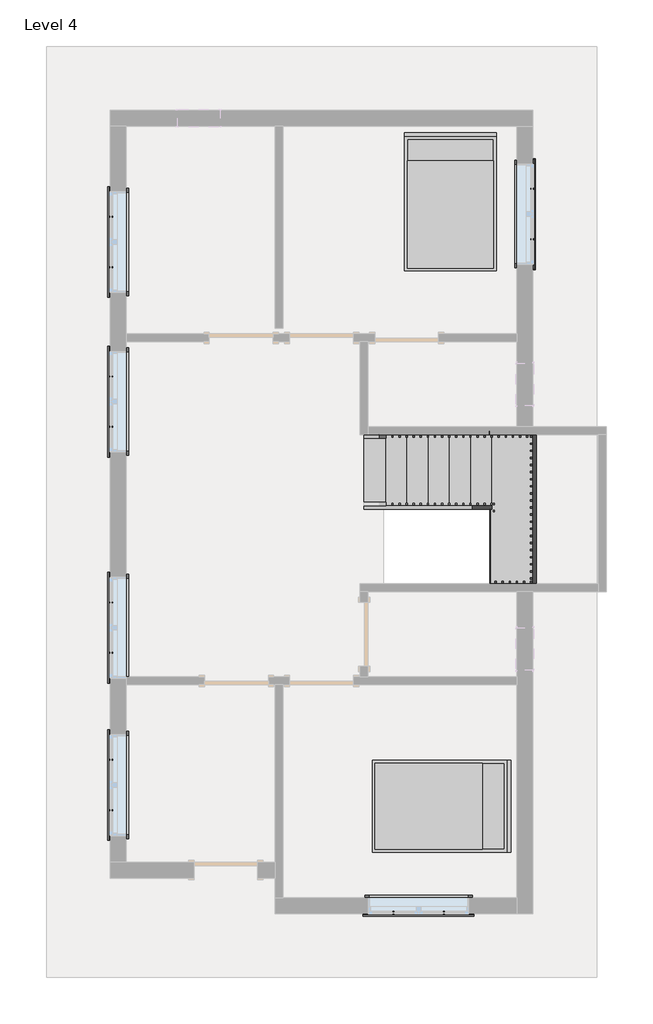
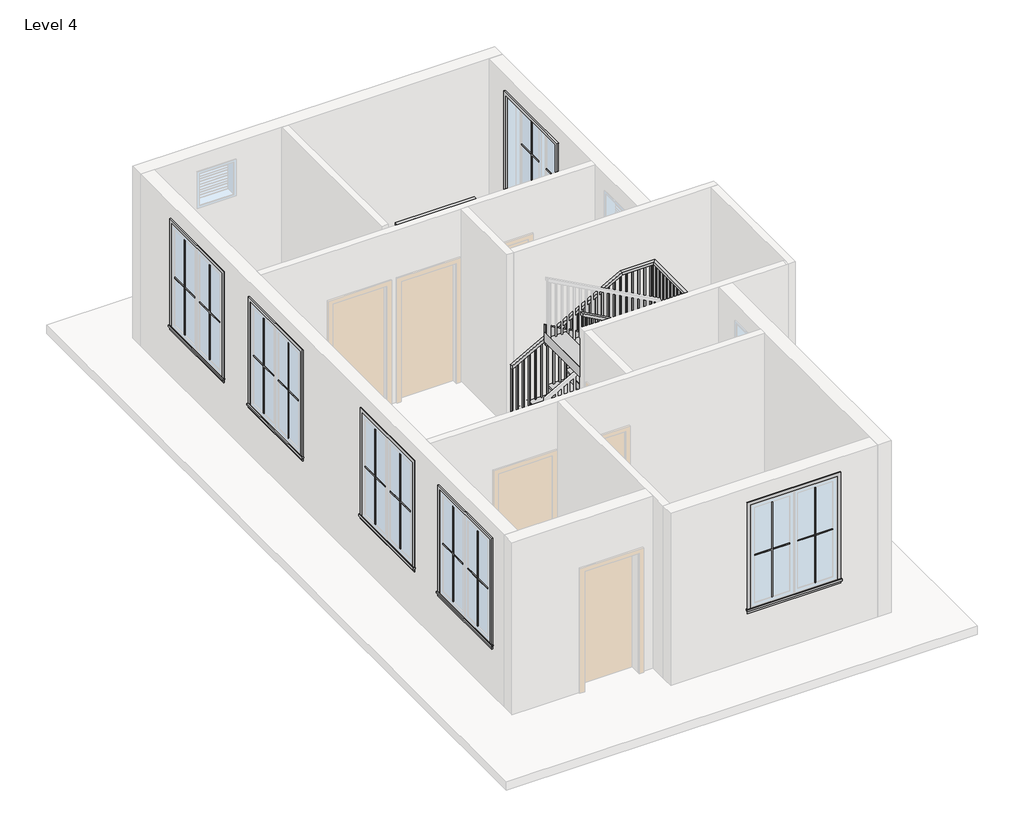
# One storey, part 2 of 2: 24 proxies, 5 members, 2 furniture elements, 1 railing, 1 stair flight.
"""IFC4 building model written with IfcOpenShell, lengths in millimetres."""

from ifc_helpers import new_model, si_unit, frame, origin, place, context, project, spatial, polyline, outline, extrude, faceted_brep, transform, mapped, element, save
from components import muntin_pattern_2x2_muntin_pattern_2x2_bff912c5, muntin_pattern_2x2_muntin_pattern_2x2_c2194282, trim_window_exterior_flat_with_sill_e04b3088, trim_window_interior_flat_picture_frame_2a7685fe, bed_17739_bed_17739_15c61121, stair_flight_c67f7d23

model = new_model("IFC4")

# Units and contexts
model_context = context("Model", 3, world=origin())
ifc_project = project(units=[si_unit("LENGTHUNIT", "METRE", prefix="MILLI")], contexts=[model_context])

# Site, building, storey
site = spatial("IfcSite", under=ifc_project)
building = spatial("IfcBuilding", under=site)
storey = spatial("IfcBuildingStorey", under=building, Name="Level 4", Elevation=6400.8)

# Proxies
placement = place(None, origin())
muntin_pattern_2x2_muntin_pattern_2x2_shape = muntin_pattern_2x2_muntin_pattern_2x2_bff912c5(model_context)
element("IfcBuildingElementProxy", 1, Name="Muntin Pattern_2x2 : Muntin Pattern_2x2", ObjectType="Muntin Pattern_2x2 : Muntin Pattern_2x2", at=placement, inside=storey, context=model_context, shape_type="MappedRepresentation", body=[
    mapped(muntin_pattern_2x2_muntin_pattern_2x2_shape, transform((-4796.6888307, -4528.6107799, 7385.05), x_axis=(0.0, 1.0, 0.0), y_axis=(-1.0, 0.0, 0.0), z_axis=(0.0, 0.0, 1.0))),
])
element("IfcBuildingElementProxy", 2, Name="Muntin Pattern_2x2 : Muntin Pattern_2x2", ObjectType="Muntin Pattern_2x2 : Muntin Pattern_2x2", at=placement, inside=storey, context=model_context, shape_type="MappedRepresentation", body=[
    mapped(muntin_pattern_2x2_muntin_pattern_2x2_shape, transform((-4796.6888307, -2274.3607799, 7385.05), x_axis=(0.0, 1.0, 0.0), y_axis=(-1.0, 0.0, 0.0), z_axis=(0.0, 0.0, 1.0))),
])
element("IfcBuildingElementProxy", 3, Name="Muntin Pattern_2x2 : Muntin Pattern_2x2", ObjectType="Muntin Pattern_2x2 : Muntin Pattern_2x2", at=placement, inside=storey, context=model_context, shape_type="MappedRepresentation", body=[
    mapped(muntin_pattern_2x2_muntin_pattern_2x2_shape, transform((-26.2513307, -6000.2232799, 7385.05), x_axis=(-1.0, 0.0, 0.0), y_axis=(0.0, -1.0, 0.0), z_axis=(0.0, 0.0, 1.0))),
])
element("IfcBuildingElementProxy", 4, Name="Muntin Pattern_2x2 : Muntin Pattern_2x2", ObjectType="Muntin Pattern_2x2 : Muntin Pattern_2x2", at=placement, inside=storey, context=model_context, shape_type="MappedRepresentation", body=[
    mapped(muntin_pattern_2x2_muntin_pattern_2x2_shape, transform((1242.1611693, 4370.9142201, 7385.05), x_axis=(0.0, -1.0, 0.0), y_axis=(1.0, 0.0, 0.0), z_axis=(0.0, 0.0, 1.0))),
])
element("IfcBuildingElementProxy", 5, Name="Muntin Pattern_2x2 : Muntin Pattern_2x2", ObjectType="Muntin Pattern_2x2 : Muntin Pattern_2x2", at=placement, inside=storey, context=model_context, shape_type="MappedRepresentation", body=[
    mapped(muntin_pattern_2x2_muntin_pattern_2x2_shape, transform((-4796.6888307, 3250.1392201, 7385.05), x_axis=(0.0, 1.0, 0.0), y_axis=(-1.0, 0.0, 0.0), z_axis=(0.0, 0.0, 1.0))),
])
element("IfcBuildingElementProxy", 6, Name="Muntin Pattern_2x2 : Muntin Pattern_2x2", ObjectType="Muntin Pattern_2x2 : Muntin Pattern_2x2", at=placement, inside=storey, context=model_context, shape_type="MappedRepresentation", body=[
    mapped(muntin_pattern_2x2_muntin_pattern_2x2_shape, transform((-4796.6888307, 964.1392201, 7385.05), x_axis=(0.0, 1.0, 0.0), y_axis=(-1.0, 0.0, 0.0), z_axis=(0.0, 0.0, 1.0))),
])
muntin_pattern_2x2_muntin_pattern_2x2_2_shape = muntin_pattern_2x2_muntin_pattern_2x2_c2194282(model_context)
element("IfcBuildingElementProxy", 7, Name="Muntin Pattern_2x2 : Muntin Pattern_2x2", ObjectType="Muntin Pattern_2x2 : Muntin Pattern_2x2", at=placement, inside=storey, context=model_context, shape_type="MappedRepresentation", body=[
    mapped(muntin_pattern_2x2_muntin_pattern_2x2_2_shape, transform((-4796.6888307, -3807.8857799, 7385.05), x_axis=(0.0, -1.0, 0.0), y_axis=(1.0, 0.0, 0.0), z_axis=(0.0, 0.0, 1.0))),
])
element("IfcBuildingElementProxy", 8, Name="Muntin Pattern_2x2 : Muntin Pattern_2x2", ObjectType="Muntin Pattern_2x2 : Muntin Pattern_2x2", at=placement, inside=storey, context=model_context, shape_type="MappedRepresentation", body=[
    mapped(muntin_pattern_2x2_muntin_pattern_2x2_2_shape, transform((-4796.6888307, -1553.6357799, 7385.05), x_axis=(0.0, -1.0, 0.0), y_axis=(1.0, 0.0, 0.0), z_axis=(0.0, 0.0, 1.0))),
])
element("IfcBuildingElementProxy", 9, Name="Muntin Pattern_2x2 : Muntin Pattern_2x2", ObjectType="Muntin Pattern_2x2 : Muntin Pattern_2x2", at=placement, inside=storey, context=model_context, shape_type="MappedRepresentation", body=[
    mapped(muntin_pattern_2x2_muntin_pattern_2x2_2_shape, transform((-746.9763307, -6000.2232799, 7385.05), x_axis=(1.0, 0.0, 0.0), y_axis=(0.0, 1.0, 0.0), z_axis=(0.0, 0.0, 1.0))),
])
element("IfcBuildingElementProxy", 10, Name="Muntin Pattern_2x2 : Muntin Pattern_2x2", ObjectType="Muntin Pattern_2x2 : Muntin Pattern_2x2", at=placement, inside=storey, context=model_context, shape_type="MappedRepresentation", body=[
    mapped(muntin_pattern_2x2_muntin_pattern_2x2_2_shape, transform((1242.1611693, 3650.1892201, 7385.05), x_axis=(0.0, 1.0, 0.0), y_axis=(-1.0, 0.0, 0.0), z_axis=(0.0, 0.0, 1.0))),
])
element("IfcBuildingElementProxy", 11, Name="Muntin Pattern_2x2 : Muntin Pattern_2x2", ObjectType="Muntin Pattern_2x2 : Muntin Pattern_2x2", at=placement, inside=storey, context=model_context, shape_type="MappedRepresentation", body=[
    mapped(muntin_pattern_2x2_muntin_pattern_2x2_2_shape, transform((-4796.6888307, 3970.8642201, 7385.05), x_axis=(0.0, -1.0, 0.0), y_axis=(1.0, 0.0, 0.0), z_axis=(0.0, 0.0, 1.0))),
])
element("IfcBuildingElementProxy", 12, Name="Muntin Pattern_2x2 : Muntin Pattern_2x2", ObjectType="Muntin Pattern_2x2 : Muntin Pattern_2x2", at=placement, inside=storey, context=model_context, shape_type="MappedRepresentation", body=[
    mapped(muntin_pattern_2x2_muntin_pattern_2x2_2_shape, transform((-4796.6888307, 1684.8642201, 7385.05), x_axis=(0.0, -1.0, 0.0), y_axis=(1.0, 0.0, 0.0), z_axis=(0.0, 0.0, 1.0))),
])
trim_window_exterior_flat_with_sill_shape = trim_window_exterior_flat_with_sill_e04b3088(model_context)
element("IfcBuildingElementProxy", 13, Name="Trim-Window-Exterior-Flat : with Sill", ObjectType="Trim-Window-Exterior-Flat : with Sill", at=placement, inside=storey, context=model_context, shape_type="MappedRepresentation", body=[
    mapped(trim_window_exterior_flat_with_sill_shape, transform((-4806.2138307, -4168.2482799, 9144.0), x_axis=(0.0, -1.0, 0.0), y_axis=(0.0, 0.0, 1.0), z_axis=(-1.0, 0.0, 0.0))),
])
element("IfcBuildingElementProxy", 14, Name="Trim-Window-Exterior-Flat : with Sill", ObjectType="Trim-Window-Exterior-Flat : with Sill", at=placement, inside=storey, context=model_context, shape_type="MappedRepresentation", body=[
    mapped(trim_window_exterior_flat_with_sill_shape, transform((-4806.2138307, -1913.9982799, 9144.0), x_axis=(0.0, -1.0, 0.0), y_axis=(0.0, 0.0, 1.0), z_axis=(-1.0, 0.0, 0.0))),
])
element("IfcBuildingElementProxy", 15, Name="Trim-Window-Exterior-Flat : with Sill", ObjectType="Trim-Window-Exterior-Flat : with Sill", at=placement, inside=storey, context=model_context, shape_type="MappedRepresentation", body=[
    mapped(trim_window_exterior_flat_with_sill_shape, transform((-386.6138307, -6009.7482799, 9144.0), x_axis=(1.0, 0.0, 0.0), y_axis=(0.0, 0.0, 1.0), z_axis=(0.0, -1.0, 0.0))),
])
element("IfcBuildingElementProxy", 16, Name="Trim-Window-Exterior-Flat : with Sill", ObjectType="Trim-Window-Exterior-Flat : with Sill", at=placement, inside=storey, context=model_context, shape_type="MappedRepresentation", body=[
    mapped(trim_window_exterior_flat_with_sill_shape, transform((1251.6861693, 4010.5517201, 9144.0), x_axis=(0.0, 1.0, 0.0), y_axis=(0.0, 0.0, 1.0), z_axis=(1.0, 0.0, 0.0))),
])
element("IfcBuildingElementProxy", 17, Name="Trim-Window-Exterior-Flat : with Sill", ObjectType="Trim-Window-Exterior-Flat : with Sill", at=placement, inside=storey, context=model_context, shape_type="MappedRepresentation", body=[
    mapped(trim_window_exterior_flat_with_sill_shape, transform((-4806.2138307, 3610.5017201, 9144.0), x_axis=(0.0, -1.0, 0.0), y_axis=(0.0, 0.0, 1.0), z_axis=(-1.0, 0.0, 0.0))),
])
element("IfcBuildingElementProxy", 18, Name="Trim-Window-Exterior-Flat : with Sill", ObjectType="Trim-Window-Exterior-Flat : with Sill", at=placement, inside=storey, context=model_context, shape_type="MappedRepresentation", body=[
    mapped(trim_window_exterior_flat_with_sill_shape, transform((-4806.2138307, 1324.5017201, 9144.0), x_axis=(0.0, -1.0, 0.0), y_axis=(0.0, 0.0, 1.0), z_axis=(-1.0, 0.0, 0.0))),
])
trim_window_interior_flat_picture_frame_shape = trim_window_interior_flat_picture_frame_2a7685fe(model_context)
element("IfcBuildingElementProxy", 19, Name="Trim-Window-Interior-Flat : Picture Frame", ObjectType="Trim-Window-Interior-Flat : Picture Frame", at=placement, inside=storey, context=model_context, shape_type="MappedRepresentation", body=[
    mapped(trim_window_interior_flat_picture_frame_shape, transform((-4577.6138307, -4168.2482799, 9144.0), x_axis=(0.0, 1.0, 0.0), y_axis=(0.0, 0.0, 1.0), z_axis=(1.0, 0.0, 0.0))),
])
element("IfcBuildingElementProxy", 20, Name="Trim-Window-Interior-Flat : Picture Frame", ObjectType="Trim-Window-Interior-Flat : Picture Frame", at=placement, inside=storey, context=model_context, shape_type="MappedRepresentation", body=[
    mapped(trim_window_interior_flat_picture_frame_shape, transform((-4577.6138307, -1913.9982799, 9144.0), x_axis=(0.0, 1.0, 0.0), y_axis=(0.0, 0.0, 1.0), z_axis=(1.0, 0.0, 0.0))),
])
element("IfcBuildingElementProxy", 21, Name="Trim-Window-Interior-Flat : Picture Frame", ObjectType="Trim-Window-Interior-Flat : Picture Frame", at=placement, inside=storey, context=model_context, shape_type="MappedRepresentation", body=[
    mapped(trim_window_interior_flat_picture_frame_shape, transform((-386.6138307, -5781.1482799, 9144.0), x_axis=(-1.0, 0.0, 0.0), y_axis=(0.0, 0.0, 1.0), z_axis=(0.0, 1.0, 0.0))),
])
element("IfcBuildingElementProxy", 22, Name="Trim-Window-Interior-Flat : Picture Frame", ObjectType="Trim-Window-Interior-Flat : Picture Frame", at=placement, inside=storey, context=model_context, shape_type="MappedRepresentation", body=[
    mapped(trim_window_interior_flat_picture_frame_shape, transform((1023.0861693, 4010.5517201, 9144.0), x_axis=(0.0, -1.0, 0.0), y_axis=(0.0, 0.0, 1.0), z_axis=(-1.0, 0.0, 0.0))),
])
element("IfcBuildingElementProxy", 23, Name="Trim-Window-Interior-Flat : Picture Frame", ObjectType="Trim-Window-Interior-Flat : Picture Frame", at=placement, inside=storey, context=model_context, shape_type="MappedRepresentation", body=[
    mapped(trim_window_interior_flat_picture_frame_shape, transform((-4577.6138307, 3610.5017201, 9144.0), x_axis=(0.0, 1.0, 0.0), y_axis=(0.0, 0.0, 1.0), z_axis=(1.0, 0.0, 0.0))),
])
element("IfcBuildingElementProxy", 24, Name="Trim-Window-Interior-Flat : Picture Frame", ObjectType="Trim-Window-Interior-Flat : Picture Frame", at=placement, inside=storey, context=model_context, shape_type="MappedRepresentation", body=[
    mapped(trim_window_interior_flat_picture_frame_shape, transform((-4577.6138307, 1324.5017201, 9144.0), x_axis=(0.0, 1.0, 0.0), y_axis=(0.0, 0.0, 1.0), z_axis=(1.0, 0.0, 0.0))),
])

# Furniture
bed_17739_bed_17739_shape = bed_17739_bed_17739_15c61121(model_context)
element("IfcFurniture", 25, ObjectType="Bed_17739 : Bed_17739", at=placement, inside=storey, context=model_context, shape_type="MappedRepresentation", body=[
    mapped(bed_17739_bed_17739_shape, transform((70.5861693, 4162.9517201, 6400.8), x_axis=(1.0, 0.0, 0.0), y_axis=(0.0, 1.0, 0.0), z_axis=(0.0, 0.0, 1.0))),
])
element("IfcFurniture", 26, ObjectType="Bed_17739 : Bed_17739", at=placement, inside=storey, context=model_context, shape_type="MappedRepresentation", body=[
    mapped(bed_17739_bed_17739_shape, transform((-81.8138307, -4473.0482799, 6400.8), x_axis=(0.0, -1.0, 0.0), y_axis=(1.0, 0.0, 0.0), z_axis=(0.0, 0.0, 1.0))),
])

# Members
element("IfcMember", 27, ObjectType="Stringer - 2\" Width", at=placement, inside=storey, context=model_context, shape_type="SweptSolid", body=[
    extrude(outline(polyline([(6604.870617, -1167.6638307), (6400.8, -1167.6638307), (6400.8, -907.3693279), (7600.2752762, 1251.6861693), (7662.3333333, 1251.6861693), (7662.3333333, 735.7690587), (6604.870617, -1167.6638307)])), frame((0.0, 848.2517201, 0.0), z_axis=(0.0, 1.0, 0.0), x_axis=(0.0, 0.0, 1.0)), (0.0, 0.0, 1.0), 50.8),
])
element("IfcMember", 28, ObjectType="Stringer - 2\" Width", at=placement, inside=storey, context=model_context, shape_type="SweptSolid", body=[
    extrude(outline(polyline([(1251.6861693, 899.0517201), (1302.4861693, 899.0517201), (1302.4861693, -1285.3482799), (1251.6861693, -1285.3482799), (1251.6861693, 899.0517201)])), frame((0.0, 0.0, 7357.5333333), z_axis=(0.0, 0.0, 1.0), x_axis=(1.0, 0.0, 0.0)), (0.0, 0.0, 1.0), 304.8),
])
element("IfcMember", 29, ObjectType="Stringer - 2\" Width", at=placement, inside=storey, context=model_context, shape_type="SweptSolid", body=[
    extrude(outline(polyline([(7357.5333333, 1302.4861693), (7440.9539503, 1302.4861693), (8823.8428392, -1186.7138307), (8475.1641651, -1186.7138307), (7357.5333333, 825.0216665), (7357.5333333, 1302.4861693)])), frame((0.0, -1336.1482799, 0.0), z_axis=(0.0, 1.0, 0.0), x_axis=(0.0, 0.0, 1.0)), (0.0, 0.0, 1.0), 50.8),
])
element("IfcMember", 30, ObjectType="Stringer - 2\" Width", at=placement, inside=storey, context=model_context, shape_type="SweptSolid", body=[
    extrude(outline(polyline([(6604.870617, -1167.6638307), (6400.8, -1167.6638307), (6400.8, -907.3693279), (7247.4974984, 616.6861693), (7596.1761726, 616.6861693), (6604.870617, -1167.6638307)])), frame((0.0, -218.5482799, 0.0), z_axis=(0.0, 1.0, 0.0), x_axis=(0.0, 0.0, 1.0)), (0.0, 0.0, 1.0), 50.8),
])
element("IfcMember", 31, ObjectType="Stringer - 2\" Width", at=placement, inside=storey, context=model_context, shape_type="SweptSolid", body=[
    extrude(outline(polyline([(7445.053054, 667.4861693), (7793.7317281, 667.4861693), (8823.8428392, -1186.7138307), (8475.1641651, -1186.7138307), (7445.053054, 667.4861693)])), frame((0.0, -218.5482799, 0.0), z_axis=(0.0, 1.0, 0.0), x_axis=(0.0, 0.0, 1.0)), (0.0, 0.0, 1.0), 50.8),
])

# Railing
element("IfcRailing", 32, ObjectType="Handrail - Rectangular", at=placement, inside=storey, context=model_context, shape_type="SolidModel", body=[
    faceted_brep([(-1167.6638307, 848.2517201, 7484.5333333), (-1167.6638307, 848.2517201, 7426.4675836), (-1167.6638307, 797.4517201, 7426.4675836), (-1167.6638307, 797.4517201, 7484.5333333), (667.4861693, 848.2517201, 8500.5333333), (680.6099298, 848.2517201, 8449.7333333), (680.6099298, 797.4517201, 8449.7333333), (667.4861693, 797.4517201, 8500.5333333), (1251.6861693, 848.2517201, 8500.5333333), (1251.6861693, 848.2517201, 8449.7333333), (1200.8861693, 797.4517201, 8449.7333333), (1200.8861693, 797.4517201, 8500.5333333), (1251.6861693, -1285.3482799, 8500.5333333), (1251.6861693, -1285.3482799, 8449.7333333), (1200.8861693, -1234.5482799, 8449.7333333), (1200.8861693, -1234.5482799, 8500.5333333), (976.5195026, -1285.3482799, 8500.5333333), (963.5139215, -1285.3482799, 8449.7333333), (963.5139215, -1234.5482799, 8449.7333333), (976.5195026, -1234.5482799, 8500.5333333), (-1186.7138307, -1285.3482799, 9685.8666667), (-1186.7138307, -1234.5482799, 9685.8666667), (-1186.7138307, -1234.5482799, 9627.9403208), (-1186.7138307, -1285.3482799, 9627.9403208)], [[[0, 1, 2, 3]], [[1, 0, 4, 5]], [[2, 1, 5, 6]], [[3, 2, 6, 7]], [[0, 3, 7, 4]], [[5, 4, 8, 9]], [[6, 5, 9, 10]], [[7, 6, 10, 11]], [[4, 7, 11, 8]], [[9, 8, 12, 13]], [[10, 9, 13, 14]], [[11, 10, 14, 15]], [[8, 11, 15, 12]], [[13, 12, 16, 17]], [[14, 13, 17, 18]], [[15, 14, 18, 19]], [[12, 15, 19, 16]], [[20, 21, 22, 23]], [[17, 16, 20, 23]], [[18, 17, 23, 22]], [[19, 18, 22, 21]], [[16, 19, 21, 20]]]),
    extrude(outline(polyline([(9591.4060742, -1120.0388307), (8602.1333333, -1120.0388307), (8602.1333333, -1100.9888307), (9580.9677181, -1100.9888307), (9591.4060742, -1120.0388307)])), frame((0.0, -1269.4732799, 0.0), z_axis=(0.0, 1.0, 0.0), x_axis=(0.0, 0.0, 1.0)), (0.0, 0.0, 1.0), 19.05),
    extrude(outline(polyline([(9535.7348414, -1018.4388307), (8602.1333333, -1018.4388307), (8602.1333333, -999.3888307), (9525.2964852, -999.3888307), (9535.7348414, -1018.4388307)])), frame((0.0, -1269.4732799, 0.0), z_axis=(0.0, 1.0, 0.0), x_axis=(0.0, 0.0, 1.0)), (0.0, 0.0, 1.0), 19.05),
    extrude(outline(polyline([(9480.0636085, -916.8388307), (8602.1333333, -916.8388307), (8602.1333333, -897.7888307), (9469.6252523, -897.7888307), (9480.0636085, -916.8388307)])), frame((0.0, -1269.4732799, 0.0), z_axis=(0.0, 1.0, 0.0), x_axis=(0.0, 0.0, 1.0)), (0.0, 0.0, 1.0), 19.05),
    extrude(outline(polyline([(9424.3923756, -815.2388307), (8432.8, -815.2388307), (8432.8, -796.1888307), (9413.9540195, -796.1888307), (9424.3923756, -815.2388307)])), frame((0.0, -1269.4732799, 0.0), z_axis=(0.0, 1.0, 0.0), x_axis=(0.0, 0.0, 1.0)), (0.0, 0.0, 1.0), 19.05),
    extrude(outline(polyline([(9368.7211427, -713.6388307), (8432.8, -713.6388307), (8432.8, -694.5888307), (9358.2827866, -694.5888307), (9368.7211427, -713.6388307)])), frame((0.0, -1269.4732799, 0.0), z_axis=(0.0, 1.0, 0.0), x_axis=(0.0, 0.0, 1.0)), (0.0, 0.0, 1.0), 19.05),
    extrude(outline(polyline([(9313.0499099, -612.0388307), (8432.8, -612.0388307), (8432.8, -592.9888307), (9302.6115537, -592.9888307), (9313.0499099, -612.0388307)])), frame((0.0, -1269.4732799, 0.0), z_axis=(0.0, 1.0, 0.0), x_axis=(0.0, 0.0, 1.0)), (0.0, 0.0, 1.0), 19.05),
    extrude(outline(polyline([(9257.378677, -510.4388307), (8263.4666667, -510.4388307), (8263.4666667, -491.3888307), (9246.9403208, -491.3888307), (9257.378677, -510.4388307)])), frame((0.0, -1269.4732799, 0.0), z_axis=(0.0, 1.0, 0.0), x_axis=(0.0, 0.0, 1.0)), (0.0, 0.0, 1.0), 19.05),
    extrude(outline(polyline([(9201.7074441, -408.8388307), (8263.4666667, -408.8388307), (8263.4666667, -389.7888307), (9191.2690879, -389.7888307), (9201.7074441, -408.8388307)])), frame((0.0, -1269.4732799, 0.0), z_axis=(0.0, 1.0, 0.0), x_axis=(0.0, 0.0, 1.0)), (0.0, 0.0, 1.0), 19.05),
    extrude(outline(polyline([(9146.0362112, -307.2388307), (8263.4666667, -307.2388307), (8263.4666667, -288.1888307), (9135.5978551, -288.1888307), (9146.0362112, -307.2388307)])), frame((0.0, -1269.4732799, 0.0), z_axis=(0.0, 1.0, 0.0), x_axis=(0.0, 0.0, 1.0)), (0.0, 0.0, 1.0), 19.05),
    extrude(outline(polyline([(9090.3649784, -205.6388307), (8094.1333333, -205.6388307), (8094.1333333, -186.5888307), (9079.9266222, -186.5888307), (9090.3649784, -205.6388307)])), frame((0.0, -1269.4732799, 0.0), z_axis=(0.0, 1.0, 0.0), x_axis=(0.0, 0.0, 1.0)), (0.0, 0.0, 1.0), 19.05),
    extrude(outline(polyline([(9034.6937455, -104.0388307), (8094.1333333, -104.0388307), (8094.1333333, -84.9888307), (9024.2553893, -84.9888307), (9034.6937455, -104.0388307)])), frame((0.0, -1269.4732799, 0.0), z_axis=(0.0, 1.0, 0.0), x_axis=(0.0, 0.0, 1.0)), (0.0, 0.0, 1.0), 19.05),
    extrude(outline(polyline([(8979.0225126, -2.4388307), (8094.1333333, -2.4388307), (8094.1333333, 16.6111693), (8968.5841564, 16.6111693), (8979.0225126, -2.4388307)])), frame((0.0, -1269.4732799, 0.0), z_axis=(0.0, 1.0, 0.0), x_axis=(0.0, 0.0, 1.0)), (0.0, 0.0, 1.0), 19.05),
    extrude(outline(polyline([(8923.3512797, 99.1611693), (7924.8, 99.1611693), (7924.8, 118.2111693), (8912.9129236, 118.2111693), (8923.3512797, 99.1611693)])), frame((0.0, -1269.4732799, 0.0), z_axis=(0.0, 1.0, 0.0), x_axis=(0.0, 0.0, 1.0)), (0.0, 0.0, 1.0), 19.05),
    extrude(outline(polyline([(8867.6800469, 200.7611693), (7924.8, 200.7611693), (7924.8, 219.8111693), (8857.2416907, 219.8111693), (8867.6800469, 200.7611693)])), frame((0.0, -1269.4732799, 0.0), z_axis=(0.0, 1.0, 0.0), x_axis=(0.0, 0.0, 1.0)), (0.0, 0.0, 1.0), 19.05),
    extrude(outline(polyline([(8812.008814, 302.3611693), (7924.8, 302.3611693), (7924.8, 321.4111693), (8801.5704578, 321.4111693), (8812.008814, 302.3611693)])), frame((0.0, -1269.4732799, 0.0), z_axis=(0.0, 1.0, 0.0), x_axis=(0.0, 0.0, 1.0)), (0.0, 0.0, 1.0), 19.05),
    extrude(outline(polyline([(8756.3375811, 403.9611693), (7755.4666667, 403.9611693), (7755.4666667, 423.0111693), (8745.8992249, 423.0111693), (8756.3375811, 403.9611693)])), frame((0.0, -1269.4732799, 0.0), z_axis=(0.0, 1.0, 0.0), x_axis=(0.0, 0.0, 1.0)), (0.0, 0.0, 1.0), 19.05),
    extrude(outline(polyline([(8700.6663482, 505.5611693), (7755.4666667, 505.5611693), (7755.4666667, 524.6111693), (8690.2279921, 524.6111693), (8700.6663482, 505.5611693)])), frame((0.0, -1269.4732799, 0.0), z_axis=(0.0, 1.0, 0.0), x_axis=(0.0, 0.0, 1.0)), (0.0, 0.0, 1.0), 19.05),
    extrude(outline(polyline([(8644.9951153, 607.1611693), (7755.4666667, 607.1611693), (7755.4666667, 626.2111693), (8634.5567592, 626.2111693), (8644.9951153, 607.1611693)])), frame((0.0, -1269.4732799, 0.0), z_axis=(0.0, 1.0, 0.0), x_axis=(0.0, 0.0, 1.0)), (0.0, 0.0, 1.0), 19.05),
    extrude(outline(polyline([(8589.3238825, 708.7611693), (7586.1333333, 708.7611693), (7586.1333333, 727.8111693), (8578.8855263, 727.8111693), (8589.3238825, 708.7611693)])), frame((0.0, -1269.4732799, 0.0), z_axis=(0.0, 1.0, 0.0), x_axis=(0.0, 0.0, 1.0)), (0.0, 0.0, 1.0), 19.05),
    extrude(outline(polyline([(8533.6526496, 810.3611693), (7586.1333333, 810.3611693), (7586.1333333, 829.4111693), (8523.2142934, 829.4111693), (8533.6526496, 810.3611693)])), frame((0.0, -1269.4732799, 0.0), z_axis=(0.0, 1.0, 0.0), x_axis=(0.0, 0.0, 1.0)), (0.0, 0.0, 1.0), 19.05),
    extrude(outline(polyline([(8477.9814167, 911.9611693), (7586.1333333, 911.9611693), (7586.1333333, 931.0111693), (8467.5430606, 931.0111693), (8477.9814167, 911.9611693)])), frame((0.0, -1269.4732799, 0.0), z_axis=(0.0, 1.0, 0.0), x_axis=(0.0, 0.0, 1.0)), (0.0, 0.0, 1.0), 19.05),
    extrude(outline(polyline([(1032.6111693, -1269.4732799), (1013.5611693, -1269.4732799), (1013.5611693, -1250.4232799), (1032.6111693, -1250.4232799), (1032.6111693, -1269.4732799)])), frame((0.0, 0.0, 7586.1333333), z_axis=(0.0, 0.0, 1.0), x_axis=(1.0, 0.0, 0.0)), (0.0, 0.0, 1.0), 863.6),
    extrude(outline(polyline([(1134.2111693, -1269.4732799), (1115.1611693, -1269.4732799), (1115.1611693, -1250.4232799), (1134.2111693, -1250.4232799), (1134.2111693, -1269.4732799)])), frame((0.0, 0.0, 7586.1333333), z_axis=(0.0, 0.0, 1.0), x_axis=(1.0, 0.0, 0.0)), (0.0, 0.0, 1.0), 863.6),
    extrude(outline(polyline([(1235.8111693, -1199.6232799), (1235.8111693, -1218.6732799), (1216.7611693, -1218.6732799), (1216.7611693, -1199.6232799), (1235.8111693, -1199.6232799)])), frame((0.0, 0.0, 7586.1333333), z_axis=(0.0, 0.0, 1.0), x_axis=(1.0, 0.0, 0.0)), (0.0, 0.0, 1.0), 863.6),
    extrude(outline(polyline([(1235.8111693, -1098.0232799), (1235.8111693, -1117.0732799), (1216.7611693, -1117.0732799), (1216.7611693, -1098.0232799), (1235.8111693, -1098.0232799)])), frame((0.0, 0.0, 7586.1333333), z_axis=(0.0, 0.0, 1.0), x_axis=(1.0, 0.0, 0.0)), (0.0, 0.0, 1.0), 863.6),
    extrude(outline(polyline([(1235.8111693, -996.4232799), (1235.8111693, -1015.4732799), (1216.7611693, -1015.4732799), (1216.7611693, -996.4232799), (1235.8111693, -996.4232799)])), frame((0.0, 0.0, 7586.1333333), z_axis=(0.0, 0.0, 1.0), x_axis=(1.0, 0.0, 0.0)), (0.0, 0.0, 1.0), 863.6),
    extrude(outline(polyline([(1235.8111693, -894.8232799), (1235.8111693, -913.8732799), (1216.7611693, -913.8732799), (1216.7611693, -894.8232799), (1235.8111693, -894.8232799)])), frame((0.0, 0.0, 7586.1333333), z_axis=(0.0, 0.0, 1.0), x_axis=(1.0, 0.0, 0.0)), (0.0, 0.0, 1.0), 863.6),
    extrude(outline(polyline([(1235.8111693, -793.2232799), (1235.8111693, -812.2732799), (1216.7611693, -812.2732799), (1216.7611693, -793.2232799), (1235.8111693, -793.2232799)])), frame((0.0, 0.0, 7586.1333333), z_axis=(0.0, 0.0, 1.0), x_axis=(1.0, 0.0, 0.0)), (0.0, 0.0, 1.0), 863.6),
    extrude(outline(polyline([(1235.8111693, -691.6232799), (1235.8111693, -710.6732799), (1216.7611693, -710.6732799), (1216.7611693, -691.6232799), (1235.8111693, -691.6232799)])), frame((0.0, 0.0, 7586.1333333), z_axis=(0.0, 0.0, 1.0), x_axis=(1.0, 0.0, 0.0)), (0.0, 0.0, 1.0), 863.6),
    extrude(outline(polyline([(1235.8111693, -590.0232799), (1235.8111693, -609.0732799), (1216.7611693, -609.0732799), (1216.7611693, -590.0232799), (1235.8111693, -590.0232799)])), frame((0.0, 0.0, 7586.1333333), z_axis=(0.0, 0.0, 1.0), x_axis=(1.0, 0.0, 0.0)), (0.0, 0.0, 1.0), 863.6),
    extrude(outline(polyline([(1235.8111693, -488.4232799), (1235.8111693, -507.4732799), (1216.7611693, -507.4732799), (1216.7611693, -488.4232799), (1235.8111693, -488.4232799)])), frame((0.0, 0.0, 7586.1333333), z_axis=(0.0, 0.0, 1.0), x_axis=(1.0, 0.0, 0.0)), (0.0, 0.0, 1.0), 863.6),
    extrude(outline(polyline([(1235.8111693, -386.8232799), (1235.8111693, -405.8732799), (1216.7611693, -405.8732799), (1216.7611693, -386.8232799), (1235.8111693, -386.8232799)])), frame((0.0, 0.0, 7586.1333333), z_axis=(0.0, 0.0, 1.0), x_axis=(1.0, 0.0, 0.0)), (0.0, 0.0, 1.0), 863.6),
    extrude(outline(polyline([(1235.8111693, -285.2232799), (1235.8111693, -304.2732799), (1216.7611693, -304.2732799), (1216.7611693, -285.2232799), (1235.8111693, -285.2232799)])), frame((0.0, 0.0, 7586.1333333), z_axis=(0.0, 0.0, 1.0), x_axis=(1.0, 0.0, 0.0)), (0.0, 0.0, 1.0), 863.6),
    extrude(outline(polyline([(1235.8111693, -183.6232799), (1235.8111693, -202.6732799), (1216.7611693, -202.6732799), (1216.7611693, -183.6232799), (1235.8111693, -183.6232799)])), frame((0.0, 0.0, 7586.1333333), z_axis=(0.0, 0.0, 1.0), x_axis=(1.0, 0.0, 0.0)), (0.0, 0.0, 1.0), 863.6),
    extrude(outline(polyline([(1235.8111693, -82.0232799), (1235.8111693, -101.0732799), (1216.7611693, -101.0732799), (1216.7611693, -82.0232799), (1235.8111693, -82.0232799)])), frame((0.0, 0.0, 7586.1333333), z_axis=(0.0, 0.0, 1.0), x_axis=(1.0, 0.0, 0.0)), (0.0, 0.0, 1.0), 863.6),
    extrude(outline(polyline([(1235.8111693, 19.5767201), (1235.8111693, 0.5267201), (1216.7611693, 0.5267201), (1216.7611693, 19.5767201), (1235.8111693, 19.5767201)])), frame((0.0, 0.0, 7586.1333333), z_axis=(0.0, 0.0, 1.0), x_axis=(1.0, 0.0, 0.0)), (0.0, 0.0, 1.0), 863.6),
    extrude(outline(polyline([(1235.8111693, 121.1767201), (1235.8111693, 102.1267201), (1216.7611693, 102.1267201), (1216.7611693, 121.1767201), (1235.8111693, 121.1767201)])), frame((0.0, 0.0, 7586.1333333), z_axis=(0.0, 0.0, 1.0), x_axis=(1.0, 0.0, 0.0)), (0.0, 0.0, 1.0), 863.6),
    extrude(outline(polyline([(1235.8111693, 222.7767201), (1235.8111693, 203.7267201), (1216.7611693, 203.7267201), (1216.7611693, 222.7767201), (1235.8111693, 222.7767201)])), frame((0.0, 0.0, 7586.1333333), z_axis=(0.0, 0.0, 1.0), x_axis=(1.0, 0.0, 0.0)), (0.0, 0.0, 1.0), 863.6),
    extrude(outline(polyline([(1235.8111693, 324.3767201), (1235.8111693, 305.3267201), (1216.7611693, 305.3267201), (1216.7611693, 324.3767201), (1235.8111693, 324.3767201)])), frame((0.0, 0.0, 7586.1333333), z_axis=(0.0, 0.0, 1.0), x_axis=(1.0, 0.0, 0.0)), (0.0, 0.0, 1.0), 863.6),
    extrude(outline(polyline([(1235.8111693, 425.9767201), (1235.8111693, 406.9267201), (1216.7611693, 406.9267201), (1216.7611693, 425.9767201), (1235.8111693, 425.9767201)])), frame((0.0, 0.0, 7586.1333333), z_axis=(0.0, 0.0, 1.0), x_axis=(1.0, 0.0, 0.0)), (0.0, 0.0, 1.0), 863.6),
    extrude(outline(polyline([(1235.8111693, 527.5767201), (1235.8111693, 508.5267201), (1216.7611693, 508.5267201), (1216.7611693, 527.5767201), (1235.8111693, 527.5767201)])), frame((0.0, 0.0, 7586.1333333), z_axis=(0.0, 0.0, 1.0), x_axis=(1.0, 0.0, 0.0)), (0.0, 0.0, 1.0), 863.6),
    extrude(outline(polyline([(1235.8111693, 629.1767201), (1235.8111693, 610.1267201), (1216.7611693, 610.1267201), (1216.7611693, 629.1767201), (1235.8111693, 629.1767201)])), frame((0.0, 0.0, 7586.1333333), z_axis=(0.0, 0.0, 1.0), x_axis=(1.0, 0.0, 0.0)), (0.0, 0.0, 1.0), 863.6),
    extrude(outline(polyline([(1235.8111693, 730.7767201), (1235.8111693, 711.7267201), (1216.7611693, 711.7267201), (1216.7611693, 730.7767201), (1235.8111693, 730.7767201)])), frame((0.0, 0.0, 7586.1333333), z_axis=(0.0, 0.0, 1.0), x_axis=(1.0, 0.0, 0.0)), (0.0, 0.0, 1.0), 863.6),
    extrude(outline(polyline([(1159.6111693, 832.3767201), (1178.6611693, 832.3767201), (1178.6611693, 813.3267201), (1159.6111693, 813.3267201), (1159.6111693, 832.3767201)])), frame((0.0, 0.0, 7586.1333333), z_axis=(0.0, 0.0, 1.0), x_axis=(1.0, 0.0, 0.0)), (0.0, 0.0, 1.0), 863.6),
    extrude(outline(polyline([(1058.0111693, 832.3767201), (1077.0611693, 832.3767201), (1077.0611693, 813.3267201), (1058.0111693, 813.3267201), (1058.0111693, 832.3767201)])), frame((0.0, 0.0, 7586.1333333), z_axis=(0.0, 0.0, 1.0), x_axis=(1.0, 0.0, 0.0)), (0.0, 0.0, 1.0), 863.6),
    extrude(outline(polyline([(956.4111693, 832.3767201), (975.4611693, 832.3767201), (975.4611693, 813.3267201), (956.4111693, 813.3267201), (956.4111693, 832.3767201)])), frame((0.0, 0.0, 7586.1333333), z_axis=(0.0, 0.0, 1.0), x_axis=(1.0, 0.0, 0.0)), (0.0, 0.0, 1.0), 863.6),
    extrude(outline(polyline([(854.8111693, 832.3767201), (873.8611693, 832.3767201), (873.8611693, 813.3267201), (854.8111693, 813.3267201), (854.8111693, 832.3767201)])), frame((0.0, 0.0, 7586.1333333), z_axis=(0.0, 0.0, 1.0), x_axis=(1.0, 0.0, 0.0)), (0.0, 0.0, 1.0), 863.6),
    extrude(outline(polyline([(753.2111693, 832.3767201), (772.2611693, 832.3767201), (772.2611693, 813.3267201), (753.2111693, 813.3267201), (753.2111693, 832.3767201)])), frame((0.0, 0.0, 7586.1333333), z_axis=(0.0, 0.0, 1.0), x_axis=(1.0, 0.0, 0.0)), (0.0, 0.0, 1.0), 863.6),
    extrude(outline(polyline([(8433.6786562, 651.6111693), (7416.8, 651.6111693), (7416.8, 670.6611693), (8444.225369, 670.6611693), (8433.6786562, 651.6111693)])), frame((0.0, 813.3267201, 0.0), z_axis=(0.0, 1.0, 0.0), x_axis=(0.0, 0.0, 1.0)), (0.0, 0.0, 1.0), 19.05),
    extrude(outline(polyline([(8377.4295213, 550.0111693), (7416.8, 550.0111693), (7416.8, 569.0611693), (8387.9762341, 569.0611693), (8377.4295213, 550.0111693)])), frame((0.0, 813.3267201, 0.0), z_axis=(0.0, 1.0, 0.0), x_axis=(0.0, 0.0, 1.0)), (0.0, 0.0, 1.0), 19.05),
    extrude(outline(polyline([(8321.1803863, 448.4111693), (7416.8, 448.4111693), (7416.8, 467.4611693), (8331.7270991, 467.4611693), (8321.1803863, 448.4111693)])), frame((0.0, 813.3267201, 0.0), z_axis=(0.0, 1.0, 0.0), x_axis=(0.0, 0.0, 1.0)), (0.0, 0.0, 1.0), 19.05),
    extrude(outline(polyline([(8264.9312514, 346.8111693), (7247.4666667, 346.8111693), (7247.4666667, 365.8611693), (8275.4779642, 365.8611693), (8264.9312514, 346.8111693)])), frame((0.0, 813.3267201, 0.0), z_axis=(0.0, 1.0, 0.0), x_axis=(0.0, 0.0, 1.0)), (0.0, 0.0, 1.0), 19.05),
    extrude(outline(polyline([(8208.6821164, 245.2111693), (7247.4666667, 245.2111693), (7247.4666667, 264.2611693), (8219.2288292, 264.2611693), (8208.6821164, 245.2111693)])), frame((0.0, 813.3267201, 0.0), z_axis=(0.0, 1.0, 0.0), x_axis=(0.0, 0.0, 1.0)), (0.0, 0.0, 1.0), 19.05),
    extrude(outline(polyline([(8152.4329815, 143.6111693), (7247.4666667, 143.6111693), (7247.4666667, 162.6611693), (8162.9796943, 162.6611693), (8152.4329815, 143.6111693)])), frame((0.0, 813.3267201, 0.0), z_axis=(0.0, 1.0, 0.0), x_axis=(0.0, 0.0, 1.0)), (0.0, 0.0, 1.0), 19.05),
    extrude(outline(polyline([(8096.1838465, 42.0111693), (7078.1333333, 42.0111693), (7078.1333333, 61.0611693), (8106.7305593, 61.0611693), (8096.1838465, 42.0111693)])), frame((0.0, 813.3267201, 0.0), z_axis=(0.0, 1.0, 0.0), x_axis=(0.0, 0.0, 1.0)), (0.0, 0.0, 1.0), 19.05),
    extrude(outline(polyline([(8039.9347116, -59.5888307), (7078.1333333, -59.5888307), (7078.1333333, -40.5388307), (8050.4814244, -40.5388307), (8039.9347116, -59.5888307)])), frame((0.0, 813.3267201, 0.0), z_axis=(0.0, 1.0, 0.0), x_axis=(0.0, 0.0, 1.0)), (0.0, 0.0, 1.0), 19.05),
    extrude(outline(polyline([(7983.6855766, -161.1888307), (7078.1333333, -161.1888307), (7078.1333333, -142.1388307), (7994.2322895, -142.1388307), (7983.6855766, -161.1888307)])), frame((0.0, 813.3267201, 0.0), z_axis=(0.0, 1.0, 0.0), x_axis=(0.0, 0.0, 1.0)), (0.0, 0.0, 1.0), 19.05),
    extrude(outline(polyline([(7927.4364417, -262.7888307), (6908.8, -262.7888307), (6908.8, -243.7388307), (7937.9831545, -243.7388307), (7927.4364417, -262.7888307)])), frame((0.0, 813.3267201, 0.0), z_axis=(0.0, 1.0, 0.0), x_axis=(0.0, 0.0, 1.0)), (0.0, 0.0, 1.0), 19.05),
    extrude(outline(polyline([(7871.1873068, -364.3888307), (6908.8, -364.3888307), (6908.8, -345.3388307), (7881.7340196, -345.3388307), (7871.1873068, -364.3888307)])), frame((0.0, 813.3267201, 0.0), z_axis=(0.0, 1.0, 0.0), x_axis=(0.0, 0.0, 1.0)), (0.0, 0.0, 1.0), 19.05),
    extrude(outline(polyline([(7814.9381718, -465.9888307), (6908.8, -465.9888307), (6908.8, -446.9388307), (7825.4848846, -446.9388307), (7814.9381718, -465.9888307)])), frame((0.0, 813.3267201, 0.0), z_axis=(0.0, 1.0, 0.0), x_axis=(0.0, 0.0, 1.0)), (0.0, 0.0, 1.0), 19.05),
    extrude(outline(polyline([(7758.6890369, -567.5888307), (6739.4666667, -567.5888307), (6739.4666667, -548.5388307), (7769.2357497, -548.5388307), (7758.6890369, -567.5888307)])), frame((0.0, 813.3267201, 0.0), z_axis=(0.0, 1.0, 0.0), x_axis=(0.0, 0.0, 1.0)), (0.0, 0.0, 1.0), 19.05),
    extrude(outline(polyline([(7702.4399019, -669.1888307), (6739.4666667, -669.1888307), (6739.4666667, -650.1388307), (7712.9866147, -650.1388307), (7702.4399019, -669.1888307)])), frame((0.0, 813.3267201, 0.0), z_axis=(0.0, 1.0, 0.0), x_axis=(0.0, 0.0, 1.0)), (0.0, 0.0, 1.0), 19.05),
    extrude(outline(polyline([(7646.190767, -770.7888307), (6739.4666667, -770.7888307), (6739.4666667, -751.7388307), (7656.7374798, -751.7388307), (7646.190767, -770.7888307)])), frame((0.0, 813.3267201, 0.0), z_axis=(0.0, 1.0, 0.0), x_axis=(0.0, 0.0, 1.0)), (0.0, 0.0, 1.0), 19.05),
    extrude(outline(polyline([(7589.941632, -872.3888307), (6570.1333333, -872.3888307), (6570.1333333, -853.3388307), (7600.4883448, -853.3388307), (7589.941632, -872.3888307)])), frame((0.0, 813.3267201, 0.0), z_axis=(0.0, 1.0, 0.0), x_axis=(0.0, 0.0, 1.0)), (0.0, 0.0, 1.0), 19.05),
    extrude(outline(polyline([(7533.6924971, -973.9888307), (6570.1333333, -973.9888307), (6570.1333333, -954.9388307), (7544.2392099, -954.9388307), (7533.6924971, -973.9888307)])), frame((0.0, 813.3267201, 0.0), z_axis=(0.0, 1.0, 0.0), x_axis=(0.0, 0.0, 1.0)), (0.0, 0.0, 1.0), 19.05),
    extrude(outline(polyline([(7477.4433621, -1075.5888307), (6570.1333333, -1075.5888307), (6570.1333333, -1056.5388307), (7487.9900749, -1056.5388307), (7477.4433621, -1075.5888307)])), frame((0.0, 813.3267201, 0.0), z_axis=(0.0, 1.0, 0.0), x_axis=(0.0, 0.0, 1.0)), (0.0, 0.0, 1.0), 19.05),
    extrude(outline(polyline([(1235.8111693, -1250.4232799), (1235.8111693, -1269.4732799), (1216.7611693, -1269.4732799), (1216.7611693, -1250.4232799), (1235.8111693, -1250.4232799)])), frame((0.0, 0.0, 7586.1333333), z_axis=(0.0, 0.0, 1.0), x_axis=(1.0, 0.0, 0.0)), (0.0, 0.0, 1.0), 863.6),
    extrude(outline(polyline([(1216.7611693, 832.3767201), (1235.8111693, 832.3767201), (1235.8111693, 813.3267201), (1216.7611693, 813.3267201), (1216.7611693, 832.3767201)])), frame((0.0, 0.0, 7586.1333333), z_axis=(0.0, 0.0, 1.0), x_axis=(1.0, 0.0, 0.0)), (0.0, 0.0, 1.0), 863.6),
    extrude(outline(polyline([(9627.9403208, -1186.7138307), (8602.1333333, -1186.7138307), (8602.1333333, -1167.6638307), (9617.5019647, -1167.6638307), (9627.9403208, -1186.7138307)])), frame((0.0, -1269.4732799, 0.0), z_axis=(0.0, 1.0, 0.0), x_axis=(0.0, 0.0, 1.0)), (0.0, 0.0, 1.0), 19.05),
    extrude(outline(polyline([(7426.4675836, -1167.6638307), (6570.1333333, -1167.6638307), (6570.1333333, -1148.6138307), (7437.0142964, -1148.6138307), (7426.4675836, -1167.6638307)])), frame((0.0, 813.3267201, 0.0), z_axis=(0.0, 1.0, 0.0), x_axis=(0.0, 0.0, 1.0)), (0.0, 0.0, 1.0), 19.05),
])

# Stair flight
stair_flight_shape = stair_flight_c67f7d23(model_context)
element("IfcStairFlight", 33, ObjectType="2\" Tread 1\" Nosing 1/4\" Riser", at=placement, inside=storey, context=model_context, shape_type="MappedRepresentation", body=[
    mapped(stair_flight_shape, transform((0.0, 0.0, 0.0), x_axis=(1.0, 0.0, 0.0), y_axis=(0.0, 1.0, 0.0), z_axis=(0.0, 0.0, 1.0))),
])

save(model, "model.ifc")

# Revit data of these elements
# Type "Muntin Pattern_2x2 : Muntin Pattern_2x2"
#   Width [instance default] = 4' - 0"
#   Thickness = 0' - 0 1/2"
#   Height [instance default] = 4' - 0"
#   Distance = 0' - 0 3/4"
#   Interior Material [instance default] = none
#   Exterior Material [instance default] = none
#   Default Elevation = 0
# Type "Trim-Window-Exterior-Flat : with Sill"
#   Trim Width = 0' - 2 1/4"
#   Trim Thickness_Picture Frame = 0' - 1 1/4"
#   Trim Thickness_with Sill = 0' - 0 3/4"
#   Sill Thickness = 0' - 1 1/4"
#   Opening Width [instance default] = 2' - 0"
#   Opening Height [instance default] = 3' - 0"
#   Default Elevation = 4' - 0"
#   Sill = yes
#   Picture Frame = no
#   Trim Material [instance default] = none
# Type "Trim-Window-Interior-Flat : Picture Frame"
#   Trim Thickness_Picture Frame = 0' - 1 1/4"
#   Trim Width = 0' - 2 1/4"
#   Trim Thickness_with Sill = 0' - 0 3/4"
#   Sill Thickness = 0' - 1 1/4"
#   Opening Width [instance default] = 2' - 0"
#   Opening Height [instance default] = 3' - 0"
#   Default Elevation = 4' - 0"
#   Sill = no
#   Picture Frame = yes
#   Trim Material [instance default] = none
# Type "Bed_17739 : Bed_17739"
#   Default Elevation = 0
# Type "Handrail - Rectangular"
#   Assembly Code = "C2010400"
#   built-in parameter 1008612 = 0.0416667 (stored number, unit not read)
#   built-in parameter 1008611 = 0.0416667 (stored number, unit not read)
#   built-in parameter 1008609 = 0.333333 (stored number, unit not read)
#   built-in parameter 1008604 = 0.166667 (stored number, unit not read)
#   built-in parameter 1008603 = 0.166667 (stored number, unit not read)
#   Railing Height = 3' - 0"
#   built-in parameter 1008630 = 2
#   built-in parameter 1008610 = 2
#   built-in parameter 1008618 = Baluster - Square : 3/4"
# Elements 1, 2, 3, 4, 5, 6, 7, 8, 9, 10, 11, 12 (IfcBuildingElementProxy, "Muntin Pattern_2x2 : Muntin Pattern_2x2")
#   Width = 1' - 11 1/8"
#   Height = 5' - 6 1/2"
#   Interior Material = Wood - Stained
#   Exterior Material = Clad - White
#   Phase Created = New Construction
#   Materials on its faces: "Clad - White", "Wood - Stained"
# Elements 13, 14, 15, 16, 17, 18 (IfcBuildingElementProxy, "Trim-Window-Exterior-Flat : with Sill")
#   Opening Width = 4' - 9"
#   Opening Height = 6' - 0"
#   Trim Material = Clad - White
#   Phase Created = New Construction
#   Materials on its faces: "Clad - White"
# Elements 19, 20, 21, 22, 23, 24 (IfcBuildingElementProxy, "Trim-Window-Interior-Flat : Picture Frame")
#   Opening Width = 4' - 9"
#   Opening Height = 6' - 0"
#   Trim Material = Wood - Stained
#   Phase Created = New Construction
#   Materials on its faces: "Wood - Stained"
# Elements 25, 26 (IfcFurniture, "Bed_17739 : Bed_17739")
#   Phase Created = New Construction
#   Materials on its faces: "legs", "sheets", "bed frame", "Blanket"
# Elements 27, 28, 29, 30, 31 (IfcMember, "Stringer - 2\" Width")
#   Phase Created = New Construction
# Element 32 (IfcRailing, "Handrail - Rectangular")
#   Phase Created = New Construction
# Element 33 (IfcStairFlight, "2\" Tread 1\" Nosing 1/4\" Riser")
#   Phase Created = New Construction
# Materials
#   "Clad - White": class "Wood", colour RGB 242 242 238, transparency 0, Cost = 0
#   "Wood - Stained": class "Wood", colour RGB 224 178 126, transparency 0, Cost = 0
#   "legs": colour RGB 90 73 37, transparency 0, Cost = 0
#   "sheets": colour RGB 200 195 176, transparency 0, Cost = 0
#   "bed frame": colour RGB 90 73 37, transparency 0, Cost = 0
#   "Blanket": class "System", colour RGB 59 0 1, transparency 0, Cost = 0
